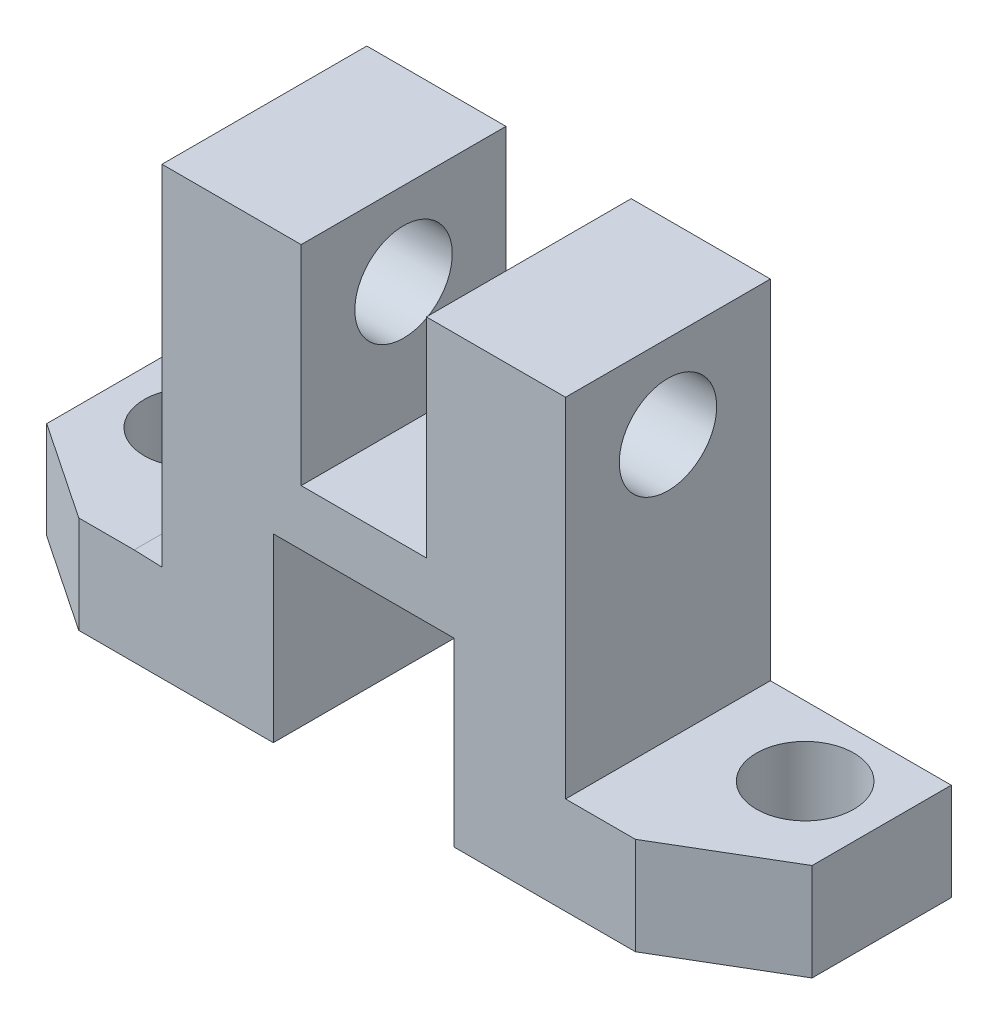
ISO-10303-21;
HEADER;
FILE_DESCRIPTION(('STEP AP214'),'2;1');
FILE_NAME('part.step','',(''),(''),'','','');
FILE_SCHEMA(('AUTOMOTIVE_DESIGN { 1 0 10303 214 1 1 1 1 }'));
ENDSEC;
DATA;
#1=APPLICATION_CONTEXT('core data for automotive mechanical design processes');
#2=APPLICATION_PROTOCOL_DEFINITION('international standard','automotive_design',2000,#1);
#3=PRODUCT_CONTEXT('',#1,'mechanical');
#4=PRODUCT('Part','Part','',(#3));
#5=PRODUCT_RELATED_PRODUCT_CATEGORY('part','',(#4));
#6=PRODUCT_DEFINITION_FORMATION('','',#4);
#7=PRODUCT_DEFINITION_CONTEXT('part definition',#1,'design');
#8=PRODUCT_DEFINITION('design','',#6,#7);
#9=PRODUCT_DEFINITION_SHAPE('','',#8);
#10=(LENGTH_UNIT() NAMED_UNIT(*) SI_UNIT(.MILLI.,.METRE.));
#11=(NAMED_UNIT(*) PLANE_ANGLE_UNIT() SI_UNIT($,.RADIAN.));
#12=(NAMED_UNIT(*) SI_UNIT($,.STERADIAN.) SOLID_ANGLE_UNIT());
#13=UNCERTAINTY_MEASURE_WITH_UNIT(LENGTH_MEASURE(1.E-05),#10,'distance_accuracy_value','');
#14=(GEOMETRIC_REPRESENTATION_CONTEXT(3) GLOBAL_UNCERTAINTY_ASSIGNED_CONTEXT((#13)) GLOBAL_UNIT_ASSIGNED_CONTEXT((#10,
#11,#12)) REPRESENTATION_CONTEXT('',''));
#15=CARTESIAN_POINT('',(0.,0.,0.));
#16=DIRECTION('',(0.,0.,1.));
#17=DIRECTION('',(1.,0.,0.));
#18=AXIS2_PLACEMENT_3D('',#15,#16,#17);
#19=CARTESIAN_POINT('',(-6.5,28.5,-8.));
#20=DIRECTION('',(0.,1.,0.));
#21=DIRECTION('',(-1.,0.,0.));
#22=AXIS2_PLACEMENT_3D('',#19,#20,#21);
#23=PLANE('',#22);
#24=DIRECTION('',(-1.,0.,0.));
#25=VECTOR('',#24,1.);
#26=CARTESIAN_POINT('',(-6.5,28.5,-8.));
#27=LINE('',#26,#25);
#28=CARTESIAN_POINT('',(-4.5,28.5,-8.));
#29=VERTEX_POINT('',#28);
#30=CARTESIAN_POINT('',(-14.5,28.5,-8.));
#31=VERTEX_POINT('',#30);
#32=EDGE_CURVE('E312',#29,#31,#27,.T.);
#33=ORIENTED_EDGE('',*,*,#32,.T.);
#34=DIRECTION('',(0.,0.,1.));
#35=VECTOR('',#34,1.);
#36=CARTESIAN_POINT('',(-14.5,28.5,-8.));
#37=LINE('',#36,#35);
#38=CARTESIAN_POINT('',(-14.5,28.5,6.71715558215924));
#39=VERTEX_POINT('',#38);
#40=EDGE_CURVE('E183',#31,#39,#37,.T.);
#41=ORIENTED_EDGE('',*,*,#40,.T.);
#42=DIRECTION('',(-1.,0.,0.));
#43=VECTOR('',#42,1.);
#44=CARTESIAN_POINT('',(-6.5,28.5,6.71715558215924));
#45=LINE('',#44,#43);
#46=CARTESIAN_POINT('',(-4.5,28.5,6.71715558215924));
#47=VERTEX_POINT('',#46);
#48=EDGE_CURVE('E310',#47,#39,#45,.T.);
#49=ORIENTED_EDGE('',*,*,#48,.F.);
#50=DIRECTION('',(0.,0.,1.));
#51=VECTOR('',#50,1.);
#52=CARTESIAN_POINT('',(-4.5,28.5,-8.));
#53=LINE('',#52,#51);
#54=EDGE_CURVE('E245',#29,#47,#53,.T.);
#55=ORIENTED_EDGE('',*,*,#54,.F.);
#56=EDGE_LOOP('',(#33,#41,#49,#55));
#57=FACE_BOUND('',#56,.T.);
#58=ADVANCED_FACE('F43',(#57),#23,.T.);
#59=CARTESIAN_POINT('',(0.,3.5,6.71715558215924));
#60=DIRECTION('',(0.,0.,-1.));
#61=DIRECTION('',(-1.,0.,0.));
#62=AXIS2_PLACEMENT_3D('',#59,#60,#61);
#63=PLANE('',#62);
#64=DIRECTION('',(-0.999304241435083,0.0372965554690129,0.));
#65=VECTOR('',#64,1.);
#66=CARTESIAN_POINT('',(0.107495075926285,2.88016638415231,6.71715558215924));
#67=LINE('',#66,#65);
#68=CARTESIAN_POINT('',(-14.5,3.42535495413198,6.71715558215924));
#69=VERTEX_POINT('',#68);
#70=CARTESIAN_POINT('',(-16.5,3.5,6.71715558215924));
#71=VERTEX_POINT('',#70);
#72=EDGE_CURVE('E192',#69,#71,#67,.T.);
#73=ORIENTED_EDGE('',*,*,#72,.T.);
#74=DIRECTION('',(1.,0.,0.));
#75=VECTOR('',#74,1.);
#76=CARTESIAN_POINT('',(0.,3.5,6.71715558215924));
#77=LINE('',#76,#75);
#78=CARTESIAN_POINT('',(-20.480974442812,3.5,6.71715558215924));
#79=VERTEX_POINT('',#78);
#80=EDGE_CURVE('E329',#79,#71,#77,.T.);
#81=ORIENTED_EDGE('',*,*,#80,.F.);
#82=DIRECTION('',(0.,-1.,0.));
#83=VECTOR('',#82,1.);
#84=CARTESIAN_POINT('',(-20.480974442812,3.5,6.71715558215924));
#85=LINE('',#84,#83);
#86=CARTESIAN_POINT('',(-20.480974442812,-3.5,6.71715558215924));
#87=VERTEX_POINT('',#86);
#88=EDGE_CURVE('E318',#79,#87,#85,.T.);
#89=ORIENTED_EDGE('',*,*,#88,.T.);
#90=DIRECTION('',(1.,0.,0.));
#91=VECTOR('',#90,1.);
#92=CARTESIAN_POINT('',(0.,-3.5,6.71715558215924));
#93=LINE('',#92,#91);
#94=CARTESIAN_POINT('',(-6.5,-3.5,6.71715558215924));
#95=VERTEX_POINT('',#94);
#96=EDGE_CURVE('E325',#87,#95,#93,.T.);
#97=ORIENTED_EDGE('',*,*,#96,.T.);
#98=DIRECTION('',(0.,-1.,0.));
#99=VECTOR('',#98,1.);
#100=CARTESIAN_POINT('',(-6.5,9.5,6.71715558215924));
#101=LINE('',#100,#99);
#102=CARTESIAN_POINT('',(-6.5,9.5,6.71715558215924));
#103=VERTEX_POINT('',#102);
#104=EDGE_CURVE('E242',#103,#95,#101,.T.);
#105=ORIENTED_EDGE('',*,*,#104,.F.);
#106=DIRECTION('',(-1.,0.,0.));
#107=VECTOR('',#106,1.);
#108=CARTESIAN_POINT('',(-6.5,9.5,6.71715558215924));
#109=LINE('',#108,#107);
#110=CARTESIAN_POINT('',(6.5,9.5,6.71715558215924));
#111=VERTEX_POINT('',#110);
#112=EDGE_CURVE('E251',#111,#103,#109,.T.);
#113=ORIENTED_EDGE('',*,*,#112,.F.);
#114=DIRECTION('',(0.,1.,0.));
#115=VECTOR('',#114,1.);
#116=CARTESIAN_POINT('',(6.5,9.5,6.71715558215924));
#117=LINE('',#116,#115);
#118=CARTESIAN_POINT('',(6.5,-3.5,6.71715558215924));
#119=VERTEX_POINT('',#118);
#120=EDGE_CURVE('E263',#119,#111,#117,.T.);
#121=ORIENTED_EDGE('',*,*,#120,.F.);
#122=CARTESIAN_POINT('',(19.519025557188,-3.5,6.71715558215924));
#123=VERTEX_POINT('',#122);
#124=EDGE_CURVE('E317',#119,#123,#93,.T.);
#125=ORIENTED_EDGE('',*,*,#124,.T.);
#126=DIRECTION('',(0.,-1.,0.));
#127=VECTOR('',#126,1.);
#128=CARTESIAN_POINT('',(19.519025557188,3.5,6.71715558215924));
#129=LINE('',#128,#127);
#130=CARTESIAN_POINT('',(19.519025557188,3.5,6.71715558215924));
#131=VERTEX_POINT('',#130);
#132=EDGE_CURVE('E297',#131,#123,#129,.T.);
#133=ORIENTED_EDGE('',*,*,#132,.F.);
#134=DIRECTION('',(1.,0.,0.));
#135=VECTOR('',#134,1.);
#136=CARTESIAN_POINT('',(0.,3.5,6.71715558215924));
#137=LINE('',#136,#135);
#138=CARTESIAN_POINT('',(14.5,3.5,6.71715558215924));
#139=VERTEX_POINT('',#138);
#140=EDGE_CURVE('E283',#139,#131,#137,.T.);
#141=ORIENTED_EDGE('',*,*,#140,.F.);
#142=DIRECTION('',(0.,-1.,0.));
#143=VECTOR('',#142,1.);
#144=CARTESIAN_POINT('',(14.5,0.,6.71715558215924));
#145=LINE('',#144,#143);
#146=CARTESIAN_POINT('',(14.5,28.5,6.71715558215924));
#147=VERTEX_POINT('',#146);
#148=EDGE_CURVE('E211',#147,#139,#145,.T.);
#149=ORIENTED_EDGE('',*,*,#148,.F.);
#150=CARTESIAN_POINT('',(4.5,28.5,6.71715558215924));
#151=VERTEX_POINT('',#150);
#152=EDGE_CURVE('E58',#147,#151,#45,.T.);
#153=ORIENTED_EDGE('',*,*,#152,.T.);
#154=DIRECTION('',(0.,1.,0.));
#155=VECTOR('',#154,1.);
#156=CARTESIAN_POINT('',(4.5,28.5,6.71715558215924));
#157=LINE('',#156,#155);
#158=CARTESIAN_POINT('',(4.5,13.5,6.71715558215924));
#159=VERTEX_POINT('',#158);
#160=EDGE_CURVE('E230',#159,#151,#157,.T.);
#161=ORIENTED_EDGE('',*,*,#160,.F.);
#162=DIRECTION('',(1.,0.,0.));
#163=VECTOR('',#162,1.);
#164=CARTESIAN_POINT('',(-4.5,13.5,6.71715558215924));
#165=LINE('',#164,#163);
#166=CARTESIAN_POINT('',(-4.5,13.5,6.71715558215924));
#167=VERTEX_POINT('',#166);
#168=EDGE_CURVE('E238',#167,#159,#165,.T.);
#169=ORIENTED_EDGE('',*,*,#168,.F.);
#170=DIRECTION('',(0.,-1.,0.));
#171=VECTOR('',#170,1.);
#172=CARTESIAN_POINT('',(-4.5,28.5,6.71715558215924));
#173=LINE('',#172,#171);
#174=EDGE_CURVE('E225',#47,#167,#173,.T.);
#175=ORIENTED_EDGE('',*,*,#174,.F.);
#176=ORIENTED_EDGE('',*,*,#48,.T.);
#177=DIRECTION('',(0.,-1.,0.));
#178=VECTOR('',#177,1.);
#179=CARTESIAN_POINT('',(-14.5,0.,6.71715558215924));
#180=LINE('',#179,#178);
#181=EDGE_CURVE('E204',#39,#69,#180,.T.);
#182=ORIENTED_EDGE('',*,*,#181,.T.);
#183=EDGE_LOOP('',(#73,#81,#89,#97,#105,#113,#121,#125,#133,#141,#149,#153,#161,#169,#175,#176,#182));
#184=FACE_BOUND('',#183,.T.);
#185=ADVANCED_FACE('F44',(#184),#63,.F.);
#186=CARTESIAN_POINT('',(0.,3.5,-8.));
#187=DIRECTION('',(0.,0.,-1.));
#188=DIRECTION('',(-1.,0.,0.));
#189=AXIS2_PLACEMENT_3D('',#186,#187,#188);
#190=PLANE('',#189);
#191=DIRECTION('',(1.,0.,0.));
#192=VECTOR('',#191,1.);
#193=CARTESIAN_POINT('',(0.,3.5,-8.));
#194=LINE('',#193,#192);
#195=CARTESIAN_POINT('',(-27.5,3.5,-8.));
#196=VERTEX_POINT('',#195);
#197=CARTESIAN_POINT('',(-16.5,3.5,-8.));
#198=VERTEX_POINT('',#197);
#199=EDGE_CURVE('E202',#196,#198,#194,.T.);
#200=ORIENTED_EDGE('',*,*,#199,.T.);
#201=DIRECTION('',(-0.999304241435083,0.0372965554690129,0.));
#202=VECTOR('',#201,1.);
#203=CARTESIAN_POINT('',(0.107495075926285,2.88016638415231,-8.));
#204=LINE('',#203,#202);
#205=CARTESIAN_POINT('',(-14.5,3.42535495413198,-8.));
#206=VERTEX_POINT('',#205);
#207=EDGE_CURVE('E186',#206,#198,#204,.T.);
#208=ORIENTED_EDGE('',*,*,#207,.F.);
#209=DIRECTION('',(0.,-1.,0.));
#210=VECTOR('',#209,1.);
#211=CARTESIAN_POINT('',(-14.5,0.,-8.));
#212=LINE('',#211,#210);
#213=EDGE_CURVE('E180',#31,#206,#212,.T.);
#214=ORIENTED_EDGE('',*,*,#213,.F.);
#215=ORIENTED_EDGE('',*,*,#32,.F.);
#216=DIRECTION('',(0.,-1.,0.));
#217=VECTOR('',#216,1.);
#218=CARTESIAN_POINT('',(-4.5,28.5,-8.));
#219=LINE('',#218,#217);
#220=CARTESIAN_POINT('',(-4.5,13.5,-8.));
#221=VERTEX_POINT('',#220);
#222=EDGE_CURVE('E223',#29,#221,#219,.T.);
#223=ORIENTED_EDGE('',*,*,#222,.T.);
#224=DIRECTION('',(1.,0.,0.));
#225=VECTOR('',#224,1.);
#226=CARTESIAN_POINT('',(-4.5,13.5,-8.));
#227=LINE('',#226,#225);
#228=CARTESIAN_POINT('',(4.5,13.5,-8.));
#229=VERTEX_POINT('',#228);
#230=EDGE_CURVE('E226',#221,#229,#227,.T.);
#231=ORIENTED_EDGE('',*,*,#230,.T.);
#232=DIRECTION('',(0.,1.,0.));
#233=VECTOR('',#232,1.);
#234=CARTESIAN_POINT('',(4.5,28.5,-8.));
#235=LINE('',#234,#233);
#236=CARTESIAN_POINT('',(4.5,28.5,-8.));
#237=VERTEX_POINT('',#236);
#238=EDGE_CURVE('E235',#229,#237,#235,.T.);
#239=ORIENTED_EDGE('',*,*,#238,.T.);
#240=CARTESIAN_POINT('',(14.5,28.5,-8.));
#241=VERTEX_POINT('',#240);
#242=EDGE_CURVE('E309',#241,#237,#27,.T.);
#243=ORIENTED_EDGE('',*,*,#242,.F.);
#244=DIRECTION('',(0.,-1.,0.));
#245=VECTOR('',#244,1.);
#246=CARTESIAN_POINT('',(14.5,0.,-8.));
#247=LINE('',#246,#245);
#248=CARTESIAN_POINT('',(14.5,3.5,-8.));
#249=VERTEX_POINT('',#248);
#250=EDGE_CURVE('E206',#241,#249,#247,.T.);
#251=ORIENTED_EDGE('',*,*,#250,.T.);
#252=DIRECTION('',(1.,0.,0.));
#253=VECTOR('',#252,1.);
#254=CARTESIAN_POINT('',(0.,3.5,-8.));
#255=LINE('',#254,#253);
#256=CARTESIAN_POINT('',(27.5,3.5,-8.));
#257=VERTEX_POINT('',#256);
#258=EDGE_CURVE('E286',#249,#257,#255,.T.);
#259=ORIENTED_EDGE('',*,*,#258,.T.);
#260=DIRECTION('',(0.,-1.,0.));
#261=VECTOR('',#260,1.);
#262=CARTESIAN_POINT('',(27.5,3.5,-8.));
#263=LINE('',#262,#261);
#264=CARTESIAN_POINT('',(27.5,-3.5,-8.));
#265=VERTEX_POINT('',#264);
#266=EDGE_CURVE('E293',#257,#265,#263,.T.);
#267=ORIENTED_EDGE('',*,*,#266,.T.);
#268=DIRECTION('',(1.,0.,0.));
#269=VECTOR('',#268,1.);
#270=CARTESIAN_POINT('',(0.,-3.5,-8.));
#271=LINE('',#270,#269);
#272=CARTESIAN_POINT('',(6.5,-3.5,-8.));
#273=VERTEX_POINT('',#272);
#274=EDGE_CURVE('E333',#273,#265,#271,.T.);
#275=ORIENTED_EDGE('',*,*,#274,.F.);
#276=DIRECTION('',(0.,1.,0.));
#277=VECTOR('',#276,1.);
#278=CARTESIAN_POINT('',(6.5,9.5,-8.));
#279=LINE('',#278,#277);
#280=CARTESIAN_POINT('',(6.5,9.5,-8.));
#281=VERTEX_POINT('',#280);
#282=EDGE_CURVE('E66',#273,#281,#279,.T.);
#283=ORIENTED_EDGE('',*,*,#282,.T.);
#284=DIRECTION('',(-1.,0.,0.));
#285=VECTOR('',#284,1.);
#286=CARTESIAN_POINT('',(-6.5,9.5,-8.));
#287=LINE('',#286,#285);
#288=CARTESIAN_POINT('',(-6.5,9.5,-8.));
#289=VERTEX_POINT('',#288);
#290=EDGE_CURVE('E259',#281,#289,#287,.T.);
#291=ORIENTED_EDGE('',*,*,#290,.T.);
#292=DIRECTION('',(0.,-1.,0.));
#293=VECTOR('',#292,1.);
#294=CARTESIAN_POINT('',(-6.5,9.5,-8.));
#295=LINE('',#294,#293);
#296=CARTESIAN_POINT('',(-6.5,-3.5,-8.));
#297=VERTEX_POINT('',#296);
#298=EDGE_CURVE('E252',#289,#297,#295,.T.);
#299=ORIENTED_EDGE('',*,*,#298,.T.);
#300=CARTESIAN_POINT('',(-27.5,-3.5,-8.));
#301=VERTEX_POINT('',#300);
#302=EDGE_CURVE('E328',#301,#297,#271,.T.);
#303=ORIENTED_EDGE('',*,*,#302,.F.);
#304=DIRECTION('',(0.,-1.,0.));
#305=VECTOR('',#304,1.);
#306=CARTESIAN_POINT('',(-27.5,3.5,-8.));
#307=LINE('',#306,#305);
#308=EDGE_CURVE('E320',#196,#301,#307,.T.);
#309=ORIENTED_EDGE('',*,*,#308,.F.);
#310=EDGE_LOOP('',(#200,#208,#214,#215,#223,#231,#239,#243,#251,#259,#267,#275,#283,#291,#299,
#303,#309));
#311=FACE_BOUND('',#310,.T.);
#312=ADVANCED_FACE('F199',(#311),#190,.T.);
#313=CARTESIAN_POINT('',(-27.5,22.5,-0.64142220892038));
#314=DIRECTION('',(1.,0.,0.));
#315=DIRECTION('',(0.,0.,-1.));
#316=AXIS2_PLACEMENT_3D('',#313,#314,#315);
#317=CYLINDRICAL_SURFACE('',#316,3.5);
#318=CARTESIAN_POINT('',(-4.5,22.5,-0.64142220892038));
#319=DIRECTION('',(-1.,0.,0.));
#320=DIRECTION('',(0.,-1.,0.));
#321=AXIS2_PLACEMENT_3D('',#318,#319,#320);
#322=CIRCLE('',#321,3.5);
#323=CARTESIAN_POINT('',(-4.5,19.,-0.64142220892038));
#324=VERTEX_POINT('',#323);
#325=EDGE_CURVE('E217',#324,#324,#322,.T.);
#326=ORIENTED_EDGE('',*,*,#325,.F.);
#327=EDGE_LOOP('',(#326));
#328=FACE_BOUND('',#327,.T.);
#329=CARTESIAN_POINT('',(-14.5,22.5,-0.64142220892038));
#330=DIRECTION('',(-1.,0.,0.));
#331=DIRECTION('',(0.,-1.,0.));
#332=AXIS2_PLACEMENT_3D('',#329,#330,#331);
#333=CIRCLE('',#332,3.5);
#334=CARTESIAN_POINT('',(-14.5,19.,-0.64142220892038));
#335=VERTEX_POINT('',#334);
#336=EDGE_CURVE('E50',#335,#335,#333,.F.);
#337=ORIENTED_EDGE('',*,*,#336,.F.);
#338=EDGE_LOOP('',(#337));
#339=FACE_BOUND('',#338,.T.);
#340=ADVANCED_FACE('F360',(#328,#339),#317,.F.);
#341=CARTESIAN_POINT('',(0.,-3.5,0.));
#342=DIRECTION('',(0.,1.,0.));
#343=DIRECTION('',(0.,0.,1.));
#344=AXIS2_PLACEMENT_3D('',#341,#342,#343);
#345=PLANE('',#344);
#346=CARTESIAN_POINT('',(-22.,-3.5,-3.));
#347=DIRECTION('',(0.,1.,0.));
#348=DIRECTION('',(0.,0.,1.));
#349=AXIS2_PLACEMENT_3D('',#346,#347,#348);
#350=CIRCLE('',#349,3.5);
#351=CARTESIAN_POINT('',(-22.,-3.5,0.5));
#352=VERTEX_POINT('',#351);
#353=EDGE_CURVE('E302',#352,#352,#350,.T.);
#354=ORIENTED_EDGE('',*,*,#353,.T.);
#355=EDGE_LOOP('',(#354));
#356=FACE_BOUND('',#355,.T.);
#357=ORIENTED_EDGE('',*,*,#302,.T.);
#358=DIRECTION('',(0.,0.,1.));
#359=VECTOR('',#358,1.);
#360=CARTESIAN_POINT('',(-6.5,-3.5,-8.));
#361=LINE('',#360,#359);
#362=EDGE_CURVE('E258',#297,#95,#361,.T.);
#363=ORIENTED_EDGE('',*,*,#362,.T.);
#364=ORIENTED_EDGE('',*,*,#96,.F.);
#365=DIRECTION('',(0.829981292389203,0.,0.557791228224278));
#366=VECTOR('',#365,1.);
#367=CARTESIAN_POINT('',(-9.48201656177849,-3.5,14.1090357147682));
#368=LINE('',#367,#366);
#369=CARTESIAN_POINT('',(-27.5,-3.5,2.));
#370=VERTEX_POINT('',#369);
#371=EDGE_CURVE('E55',#370,#87,#368,.T.);
#372=ORIENTED_EDGE('',*,*,#371,.F.);
#373=DIRECTION('',(0.,0.,1.));
#374=VECTOR('',#373,1.);
#375=CARTESIAN_POINT('',(-27.5,-3.5,0.));
#376=LINE('',#375,#374);
#377=EDGE_CURVE('E319',#301,#370,#376,.T.);
#378=ORIENTED_EDGE('',*,*,#377,.F.);
#379=EDGE_LOOP('',(#357,#363,#364,#372,#378));
#380=FACE_BOUND('',#379,.T.);
#381=ADVANCED_FACE('F407',(#356,#380),#345,.F.);
#382=CARTESIAN_POINT('',(0.,3.5,0.));
#383=DIRECTION('',(0.,1.,0.));
#384=DIRECTION('',(0.,0.,1.));
#385=AXIS2_PLACEMENT_3D('',#382,#383,#384);
#386=PLANE('',#385);
#387=CARTESIAN_POINT('',(-22.,3.5,-3.));
#388=DIRECTION('',(0.,1.,0.));
#389=DIRECTION('',(0.,0.,1.));
#390=AXIS2_PLACEMENT_3D('',#387,#388,#389);
#391=CIRCLE('',#390,3.5);
#392=CARTESIAN_POINT('',(-22.,3.5,0.5));
#393=VERTEX_POINT('',#392);
#394=EDGE_CURVE('E303',#393,#393,#391,.T.);
#395=ORIENTED_EDGE('',*,*,#394,.F.);
#396=EDGE_LOOP('',(#395));
#397=FACE_BOUND('',#396,.T.);
#398=DIRECTION('',(0.,0.,1.));
#399=VECTOR('',#398,1.);
#400=CARTESIAN_POINT('',(-16.5,3.5,0.));
#401=LINE('',#400,#399);
#402=EDGE_CURVE('E315',#198,#71,#401,.T.);
#403=ORIENTED_EDGE('',*,*,#402,.F.);
#404=ORIENTED_EDGE('',*,*,#199,.F.);
#405=DIRECTION('',(0.,0.,1.));
#406=VECTOR('',#405,1.);
#407=CARTESIAN_POINT('',(-27.5,3.5,0.));
#408=LINE('',#407,#406);
#409=CARTESIAN_POINT('',(-27.5,3.5,2.));
#410=VERTEX_POINT('',#409);
#411=EDGE_CURVE('E327',#196,#410,#408,.T.);
#412=ORIENTED_EDGE('',*,*,#411,.T.);
#413=DIRECTION('',(0.829981292389203,0.,0.557791228224278));
#414=VECTOR('',#413,1.);
#415=CARTESIAN_POINT('',(-9.48201656177849,3.5,14.1090357147682));
#416=LINE('',#415,#414);
#417=EDGE_CURVE('E330',#410,#79,#416,.T.);
#418=ORIENTED_EDGE('',*,*,#417,.T.);
#419=ORIENTED_EDGE('',*,*,#80,.T.);
#420=EDGE_LOOP('',(#403,#404,#412,#418,#419));
#421=FACE_BOUND('',#420,.T.);
#422=ADVANCED_FACE('F402',(#397,#421),#386,.T.);
#423=ORIENTED_EDGE('',*,*,#124,.F.);
#424=DIRECTION('',(0.,0.,1.));
#425=VECTOR('',#424,1.);
#426=CARTESIAN_POINT('',(6.5,-3.5,-8.));
#427=LINE('',#426,#425);
#428=EDGE_CURVE('E272',#273,#119,#427,.T.);
#429=ORIENTED_EDGE('',*,*,#428,.F.);
#430=ORIENTED_EDGE('',*,*,#274,.T.);
#431=DIRECTION('',(0.,0.,-1.));
#432=VECTOR('',#431,1.);
#433=CARTESIAN_POINT('',(27.5,-3.5,0.));
#434=LINE('',#433,#432);
#435=CARTESIAN_POINT('',(27.5,-3.5,2.));
#436=VERTEX_POINT('',#435);
#437=EDGE_CURVE('E284',#436,#265,#434,.T.);
#438=ORIENTED_EDGE('',*,*,#437,.F.);
#439=DIRECTION('',(0.860873364447558,0.,-0.508819270846479));
#440=VECTOR('',#439,1.);
#441=CARTESIAN_POINT('',(7.99572680075915,-3.5,13.528002232938));
#442=LINE('',#441,#440);
#443=EDGE_CURVE('E280',#123,#436,#442,.T.);
#444=ORIENTED_EDGE('',*,*,#443,.F.);
#445=EDGE_LOOP('',(#423,#429,#430,#438,#444));
#446=FACE_BOUND('',#445,.T.);
#447=CARTESIAN_POINT('',(22.,-3.5,-3.));
#448=DIRECTION('',(0.,1.,0.));
#449=DIRECTION('',(0.,0.,1.));
#450=AXIS2_PLACEMENT_3D('',#447,#448,#449);
#451=CIRCLE('',#450,3.5);
#452=CARTESIAN_POINT('',(22.,-3.5,0.5));
#453=VERTEX_POINT('',#452);
#454=EDGE_CURVE('E273',#453,#453,#451,.F.);
#455=ORIENTED_EDGE('',*,*,#454,.F.);
#456=EDGE_LOOP('',(#455));
#457=FACE_BOUND('',#456,.T.);
#458=ADVANCED_FACE('F428',(#446,#457),#345,.F.);
#459=CARTESIAN_POINT('',(-27.5,3.5,0.));
#460=DIRECTION('',(1.,0.,0.));
#461=DIRECTION('',(0.,0.,-1.));
#462=AXIS2_PLACEMENT_3D('',#459,#460,#461);
#463=PLANE('',#462);
#464=ORIENTED_EDGE('',*,*,#377,.T.);
#465=DIRECTION('',(0.,-1.,0.));
#466=VECTOR('',#465,1.);
#467=CARTESIAN_POINT('',(-27.5,3.5,2.));
#468=LINE('',#467,#466);
#469=EDGE_CURVE('E11',#410,#370,#468,.T.);
#470=ORIENTED_EDGE('',*,*,#469,.F.);
#471=ORIENTED_EDGE('',*,*,#411,.F.);
#472=ORIENTED_EDGE('',*,*,#308,.T.);
#473=EDGE_LOOP('',(#464,#470,#471,#472));
#474=FACE_BOUND('',#473,.T.);
#475=ADVANCED_FACE('F382',(#474),#463,.F.);
#476=CARTESIAN_POINT('',(-9.48201656177849,3.5,14.1090357147682));
#477=DIRECTION('',(0.557791228224278,0.,-0.829981292389203));
#478=DIRECTION('',(-0.829981292389203,0.,-0.557791228224278));
#479=AXIS2_PLACEMENT_3D('',#476,#477,#478);
#480=PLANE('',#479);
#481=ORIENTED_EDGE('',*,*,#371,.T.);
#482=ORIENTED_EDGE('',*,*,#88,.F.);
#483=ORIENTED_EDGE('',*,*,#417,.F.);
#484=ORIENTED_EDGE('',*,*,#469,.T.);
#485=EDGE_LOOP('',(#481,#482,#483,#484));
#486=FACE_BOUND('',#485,.T.);
#487=ADVANCED_FACE('F371',(#486),#480,.F.);
#488=DIRECTION('',(0.,0.,1.));
#489=VECTOR('',#488,1.);
#490=CARTESIAN_POINT('',(14.5,28.5,-8.));
#491=LINE('',#490,#489);
#492=EDGE_CURVE('E212',#241,#147,#491,.T.);
#493=ORIENTED_EDGE('',*,*,#492,.F.);
#494=ORIENTED_EDGE('',*,*,#242,.T.);
#495=DIRECTION('',(0.,0.,1.));
#496=VECTOR('',#495,1.);
#497=CARTESIAN_POINT('',(4.5,28.5,-8.));
#498=LINE('',#497,#496);
#499=EDGE_CURVE('E244',#237,#151,#498,.T.);
#500=ORIENTED_EDGE('',*,*,#499,.T.);
#501=ORIENTED_EDGE('',*,*,#152,.F.);
#502=EDGE_LOOP('',(#493,#494,#500,#501));
#503=FACE_BOUND('',#502,.T.);
#504=ADVANCED_FACE('F361',(#503),#23,.T.);
#505=CARTESIAN_POINT('',(-22.,-3.5,-3.));
#506=DIRECTION('',(0.,1.,0.));
#507=DIRECTION('',(0.,0.,1.));
#508=AXIS2_PLACEMENT_3D('',#505,#506,#507);
#509=CYLINDRICAL_SURFACE('',#508,3.5);
#510=ORIENTED_EDGE('',*,*,#353,.F.);
#511=EDGE_LOOP('',(#510));
#512=FACE_BOUND('',#511,.T.);
#513=ORIENTED_EDGE('',*,*,#394,.T.);
#514=EDGE_LOOP('',(#513));
#515=FACE_BOUND('',#514,.T.);
#516=ADVANCED_FACE('F369',(#512,#515),#509,.F.);
#517=CARTESIAN_POINT('',(7.99572680075915,3.5,13.528002232938));
#518=DIRECTION('',(-0.508819270846479,0.,-0.860873364447558));
#519=DIRECTION('',(-0.860873364447558,0.,0.508819270846479));
#520=AXIS2_PLACEMENT_3D('',#517,#518,#519);
#521=PLANE('',#520);
#522=ORIENTED_EDGE('',*,*,#443,.T.);
#523=DIRECTION('',(0.,-1.,0.));
#524=VECTOR('',#523,1.);
#525=CARTESIAN_POINT('',(27.5,3.5,2.));
#526=LINE('',#525,#524);
#527=CARTESIAN_POINT('',(27.5,3.5,2.));
#528=VERTEX_POINT('',#527);
#529=EDGE_CURVE('E300',#528,#436,#526,.T.);
#530=ORIENTED_EDGE('',*,*,#529,.F.);
#531=DIRECTION('',(0.860873364447558,0.,-0.508819270846479));
#532=VECTOR('',#531,1.);
#533=CARTESIAN_POINT('',(7.99572680075915,3.5,13.528002232938));
#534=LINE('',#533,#532);
#535=EDGE_CURVE('E281',#131,#528,#534,.T.);
#536=ORIENTED_EDGE('',*,*,#535,.F.);
#537=ORIENTED_EDGE('',*,*,#132,.T.);
#538=EDGE_LOOP('',(#522,#530,#536,#537));
#539=FACE_BOUND('',#538,.T.);
#540=ADVANCED_FACE('F377',(#539),#521,.F.);
#541=CARTESIAN_POINT('',(27.5,3.5,0.));
#542=DIRECTION('',(-1.,0.,0.));
#543=DIRECTION('',(0.,0.,1.));
#544=AXIS2_PLACEMENT_3D('',#541,#542,#543);
#545=PLANE('',#544);
#546=ORIENTED_EDGE('',*,*,#437,.T.);
#547=ORIENTED_EDGE('',*,*,#266,.F.);
#548=DIRECTION('',(0.,0.,-1.));
#549=VECTOR('',#548,1.);
#550=CARTESIAN_POINT('',(27.5,3.5,0.));
#551=LINE('',#550,#549);
#552=EDGE_CURVE('E287',#528,#257,#551,.T.);
#553=ORIENTED_EDGE('',*,*,#552,.F.);
#554=ORIENTED_EDGE('',*,*,#529,.T.);
#555=EDGE_LOOP('',(#546,#547,#553,#554));
#556=FACE_BOUND('',#555,.T.);
#557=ADVANCED_FACE('F438',(#556),#545,.F.);
#558=CARTESIAN_POINT('',(0.,3.5,0.));
#559=DIRECTION('',(0.,1.,0.));
#560=DIRECTION('',(0.,0.,1.));
#561=AXIS2_PLACEMENT_3D('',#558,#559,#560);
#562=PLANE('',#561);
#563=CARTESIAN_POINT('',(22.,3.5,-3.));
#564=DIRECTION('',(0.,1.,0.));
#565=DIRECTION('',(0.,0.,1.));
#566=AXIS2_PLACEMENT_3D('',#563,#564,#565);
#567=CIRCLE('',#566,3.5);
#568=CARTESIAN_POINT('',(22.,3.5,0.5));
#569=VERTEX_POINT('',#568);
#570=EDGE_CURVE('E270',#569,#569,#567,.F.);
#571=ORIENTED_EDGE('',*,*,#570,.T.);
#572=EDGE_LOOP('',(#571));
#573=FACE_BOUND('',#572,.T.);
#574=ORIENTED_EDGE('',*,*,#258,.F.);
#575=DIRECTION('',(0.,0.,1.));
#576=VECTOR('',#575,1.);
#577=CARTESIAN_POINT('',(14.5,3.5,-8.));
#578=LINE('',#577,#576);
#579=EDGE_CURVE('E214',#249,#139,#578,.T.);
#580=ORIENTED_EDGE('',*,*,#579,.T.);
#581=ORIENTED_EDGE('',*,*,#140,.T.);
#582=ORIENTED_EDGE('',*,*,#535,.T.);
#583=ORIENTED_EDGE('',*,*,#552,.T.);
#584=EDGE_LOOP('',(#574,#580,#581,#582,#583));
#585=FACE_BOUND('',#584,.T.);
#586=ADVANCED_FACE('F432',(#573,#585),#562,.T.);
#587=CARTESIAN_POINT('',(22.,-3.5,-3.));
#588=DIRECTION('',(0.,1.,0.));
#589=DIRECTION('',(0.,0.,1.));
#590=AXIS2_PLACEMENT_3D('',#587,#588,#589);
#591=CYLINDRICAL_SURFACE('',#590,3.5);
#592=ORIENTED_EDGE('',*,*,#454,.T.);
#593=EDGE_LOOP('',(#592));
#594=FACE_BOUND('',#593,.T.);
#595=ORIENTED_EDGE('',*,*,#570,.F.);
#596=EDGE_LOOP('',(#595));
#597=FACE_BOUND('',#596,.T.);
#598=ADVANCED_FACE('F444',(#594,#597),#591,.F.);
#599=CARTESIAN_POINT('',(-6.5,9.5,-8.));
#600=DIRECTION('',(-1.,0.,0.));
#601=DIRECTION('',(0.,-1.,0.));
#602=AXIS2_PLACEMENT_3D('',#599,#600,#601);
#603=PLANE('',#602);
#604=ORIENTED_EDGE('',*,*,#104,.T.);
#605=ORIENTED_EDGE('',*,*,#362,.F.);
#606=ORIENTED_EDGE('',*,*,#298,.F.);
#607=DIRECTION('',(0.,0.,1.));
#608=VECTOR('',#607,1.);
#609=CARTESIAN_POINT('',(-6.5,9.5,-8.));
#610=LINE('',#609,#608);
#611=EDGE_CURVE('E267',#289,#103,#610,.T.);
#612=ORIENTED_EDGE('',*,*,#611,.T.);
#613=EDGE_LOOP('',(#604,#605,#606,#612));
#614=FACE_BOUND('',#613,.T.);
#615=ADVANCED_FACE('F412',(#614),#603,.F.);
#616=CARTESIAN_POINT('',(-6.5,9.5,-8.));
#617=DIRECTION('',(0.,1.,0.));
#618=DIRECTION('',(0.,0.,1.));
#619=AXIS2_PLACEMENT_3D('',#616,#617,#618);
#620=PLANE('',#619);
#621=ORIENTED_EDGE('',*,*,#112,.T.);
#622=ORIENTED_EDGE('',*,*,#611,.F.);
#623=ORIENTED_EDGE('',*,*,#290,.F.);
#624=DIRECTION('',(0.,0.,1.));
#625=VECTOR('',#624,1.);
#626=CARTESIAN_POINT('',(6.5,9.5,-8.));
#627=LINE('',#626,#625);
#628=EDGE_CURVE('E266',#281,#111,#627,.T.);
#629=ORIENTED_EDGE('',*,*,#628,.T.);
#630=EDGE_LOOP('',(#621,#622,#623,#629));
#631=FACE_BOUND('',#630,.T.);
#632=ADVANCED_FACE('F416',(#631),#620,.F.);
#633=CARTESIAN_POINT('',(6.5,9.5,-8.));
#634=DIRECTION('',(1.,0.,0.));
#635=DIRECTION('',(0.,1.,0.));
#636=AXIS2_PLACEMENT_3D('',#633,#634,#635);
#637=PLANE('',#636);
#638=ORIENTED_EDGE('',*,*,#120,.T.);
#639=ORIENTED_EDGE('',*,*,#628,.F.);
#640=ORIENTED_EDGE('',*,*,#282,.F.);
#641=ORIENTED_EDGE('',*,*,#428,.T.);
#642=EDGE_LOOP('',(#638,#639,#640,#641));
#643=FACE_BOUND('',#642,.T.);
#644=ADVANCED_FACE('F453',(#643),#637,.F.);
#645=CARTESIAN_POINT('',(-4.5,28.5,-8.));
#646=DIRECTION('',(-1.,0.,0.));
#647=DIRECTION('',(0.,-1.,0.));
#648=AXIS2_PLACEMENT_3D('',#645,#646,#647);
#649=PLANE('',#648);
#650=ORIENTED_EDGE('',*,*,#325,.T.);
#651=EDGE_LOOP('',(#650));
#652=FACE_BOUND('',#651,.T.);
#653=ORIENTED_EDGE('',*,*,#174,.T.);
#654=DIRECTION('',(0.,0.,1.));
#655=VECTOR('',#654,1.);
#656=CARTESIAN_POINT('',(-4.5,13.5,-8.));
#657=LINE('',#656,#655);
#658=EDGE_CURVE('E232',#221,#167,#657,.T.);
#659=ORIENTED_EDGE('',*,*,#658,.F.);
#660=ORIENTED_EDGE('',*,*,#222,.F.);
#661=ORIENTED_EDGE('',*,*,#54,.T.);
#662=EDGE_LOOP('',(#653,#659,#660,#661));
#663=FACE_BOUND('',#662,.T.);
#664=ADVANCED_FACE('F399',(#652,#663),#649,.F.);
#665=CARTESIAN_POINT('',(4.5,28.5,-8.));
#666=DIRECTION('',(1.,0.,0.));
#667=DIRECTION('',(0.,1.,0.));
#668=AXIS2_PLACEMENT_3D('',#665,#666,#667);
#669=PLANE('',#668);
#670=CARTESIAN_POINT('',(4.5,22.5,-0.64142220892038));
#671=DIRECTION('',(1.,0.,0.));
#672=DIRECTION('',(0.,1.,0.));
#673=AXIS2_PLACEMENT_3D('',#670,#671,#672);
#674=CIRCLE('',#673,3.5);
#675=CARTESIAN_POINT('',(4.5,26.,-0.64142220892038));
#676=VERTEX_POINT('',#675);
#677=EDGE_CURVE('E221',#676,#676,#674,.T.);
#678=ORIENTED_EDGE('',*,*,#677,.T.);
#679=EDGE_LOOP('',(#678));
#680=FACE_BOUND('',#679,.T.);
#681=ORIENTED_EDGE('',*,*,#160,.T.);
#682=ORIENTED_EDGE('',*,*,#499,.F.);
#683=ORIENTED_EDGE('',*,*,#238,.F.);
#684=DIRECTION('',(0.,0.,1.));
#685=VECTOR('',#684,1.);
#686=CARTESIAN_POINT('',(4.5,13.5,-8.));
#687=LINE('',#686,#685);
#688=EDGE_CURVE('E247',#229,#159,#687,.T.);
#689=ORIENTED_EDGE('',*,*,#688,.T.);
#690=EDGE_LOOP('',(#681,#682,#683,#689));
#691=FACE_BOUND('',#690,.T.);
#692=ADVANCED_FACE('F387',(#680,#691),#669,.F.);
#693=CARTESIAN_POINT('',(-4.5,13.5,-8.));
#694=DIRECTION('',(0.,-1.,0.));
#695=DIRECTION('',(0.,0.,-1.));
#696=AXIS2_PLACEMENT_3D('',#693,#694,#695);
#697=PLANE('',#696);
#698=ORIENTED_EDGE('',*,*,#168,.T.);
#699=ORIENTED_EDGE('',*,*,#688,.F.);
#700=ORIENTED_EDGE('',*,*,#230,.F.);
#701=ORIENTED_EDGE('',*,*,#658,.T.);
#702=EDGE_LOOP('',(#698,#699,#700,#701));
#703=FACE_BOUND('',#702,.T.);
#704=ADVANCED_FACE('F357',(#703),#697,.F.);
#705=CARTESIAN_POINT('',(14.5,22.5,-0.64142220892038));
#706=DIRECTION('',(-1.,0.,0.));
#707=DIRECTION('',(0.,-1.,0.));
#708=AXIS2_PLACEMENT_3D('',#705,#706,#707);
#709=CIRCLE('',#708,3.5);
#710=CARTESIAN_POINT('',(14.5,19.,-0.64142220892038));
#711=VERTEX_POINT('',#710);
#712=EDGE_CURVE('E220',#711,#711,#709,.F.);
#713=ORIENTED_EDGE('',*,*,#712,.T.);
#714=EDGE_LOOP('',(#713));
#715=FACE_BOUND('',#714,.T.);
#716=ORIENTED_EDGE('',*,*,#677,.F.);
#717=EDGE_LOOP('',(#716));
#718=FACE_BOUND('',#717,.T.);
#719=ADVANCED_FACE('F343',(#715,#718),#317,.F.);
#720=CARTESIAN_POINT('',(14.5,0.,-8.));
#721=DIRECTION('',(-1.,0.,0.));
#722=DIRECTION('',(0.,-1.,0.));
#723=AXIS2_PLACEMENT_3D('',#720,#721,#722);
#724=PLANE('',#723);
#725=ORIENTED_EDGE('',*,*,#148,.T.);
#726=ORIENTED_EDGE('',*,*,#579,.F.);
#727=ORIENTED_EDGE('',*,*,#250,.F.);
#728=ORIENTED_EDGE('',*,*,#492,.T.);
#729=EDGE_LOOP('',(#725,#726,#727,#728));
#730=FACE_BOUND('',#729,.T.);
#731=ORIENTED_EDGE('',*,*,#712,.F.);
#732=EDGE_LOOP('',(#731));
#733=FACE_BOUND('',#732,.T.);
#734=ADVANCED_FACE('F350',(#730,#733),#724,.F.);
#735=CARTESIAN_POINT('',(-14.5,0.,-8.));
#736=DIRECTION('',(-1.,0.,0.));
#737=DIRECTION('',(0.,-1.,0.));
#738=AXIS2_PLACEMENT_3D('',#735,#736,#737);
#739=PLANE('',#738);
#740=ORIENTED_EDGE('',*,*,#181,.F.);
#741=ORIENTED_EDGE('',*,*,#40,.F.);
#742=ORIENTED_EDGE('',*,*,#213,.T.);
#743=DIRECTION('',(0.,0.,1.));
#744=VECTOR('',#743,1.);
#745=CARTESIAN_POINT('',(-14.5,3.42535495413198,-8.));
#746=LINE('',#745,#744);
#747=EDGE_CURVE('E181',#206,#69,#746,.T.);
#748=ORIENTED_EDGE('',*,*,#747,.T.);
#749=EDGE_LOOP('',(#740,#741,#742,#748));
#750=FACE_BOUND('',#749,.T.);
#751=ORIENTED_EDGE('',*,*,#336,.T.);
#752=EDGE_LOOP('',(#751));
#753=FACE_BOUND('',#752,.T.);
#754=ADVANCED_FACE('F177',(#750,#753),#739,.T.);
#755=CARTESIAN_POINT('',(0.107495075926285,2.88016638415231,-8.));
#756=DIRECTION('',(0.0372965554690129,0.999304241435083,0.));
#757=DIRECTION('',(-0.999304241435083,0.0372965554690129,0.));
#758=AXIS2_PLACEMENT_3D('',#755,#756,#757);
#759=PLANE('',#758);
#760=ORIENTED_EDGE('',*,*,#72,.F.);
#761=ORIENTED_EDGE('',*,*,#747,.F.);
#762=ORIENTED_EDGE('',*,*,#207,.T.);
#763=ORIENTED_EDGE('',*,*,#402,.T.);
#764=EDGE_LOOP('',(#760,#761,#762,#763));
#765=FACE_BOUND('',#764,.T.);
#766=ADVANCED_FACE('F191',(#765),#759,.T.);
#767=CLOSED_SHELL('',(#58,#185,#312,#340,#381,#422,#458,#475,#487,#504,#516,#540,#557,#586,#598,
#615,#632,#644,#664,#692,#704,#719,#734,#754,#766));
#768=MANIFOLD_SOLID_BREP('B2',#767);
#769=ADVANCED_BREP_SHAPE_REPRESENTATION('',(#18,#768),#14);
#770=SHAPE_DEFINITION_REPRESENTATION(#9,#769);
ENDSEC;
END-ISO-10303-21;
